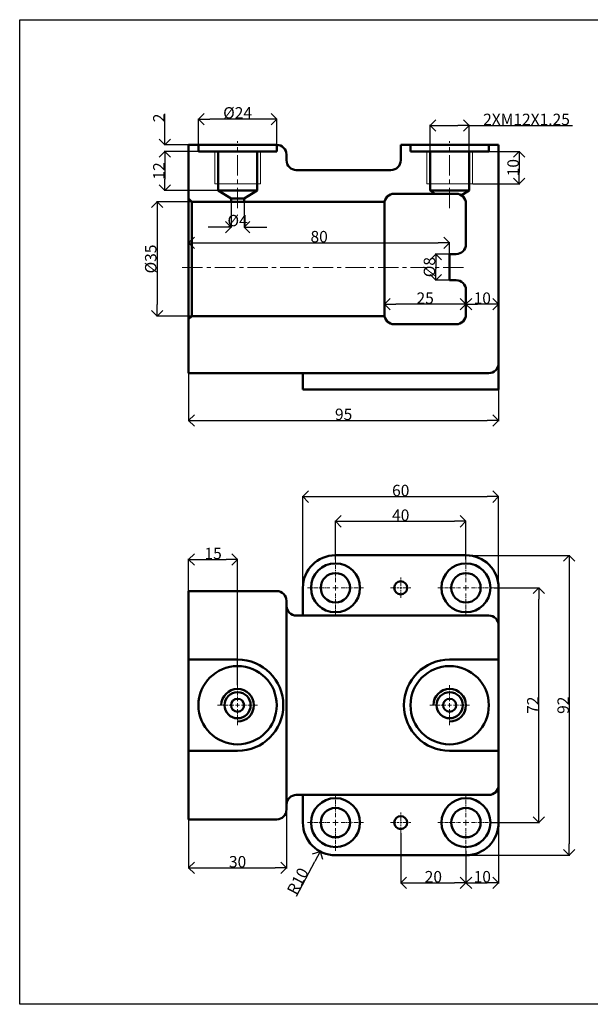
# Model space of a CAD drawing. Units: millimetres. Extents: x 47 to 397, y 26 to 328.
# Tile 1 of 2: x 47 to 222, y 26 to 328. Entities that reach past the tile are written whole.
import ezdxf

# ---------------------------------------------------------------- set-up
doc = ezdxf.new("R2010")
doc.units = ezdxf.units.MM
doc.header["$MEASUREMENT"] = 0
doc.linetypes.add('CENTER', pattern=[2, 1.25, -0.25, 0.25, -0.25])
for name, color, linetype, lineweight in [('M-CNTR', 1, 'CENTER', 18), ('M-DIMS', 2, 'Continuous', 25), ('M-OUTL', 7, 'Continuous', 50), ('M-THRD', 8, 'Continuous', 18), ('M-TTLB', 7, 'Continuous', 25)]:
    doc.layers.add(name, color=color, linetype=linetype, lineweight=lineweight)
doc.styles.get("Standard").update_dxf_attribs({"font": 'arial.ttf'})
doc.dimstyles.get("Standard").update_dxf_attribs({"dimtxt": 3.5, "dimasz": 3.5, "dimexe": 0.18, "dimexo": 0.0625, "dimgap": 0.09, "dimtad": 1, "dimdec": 0, "dimzin": 0, "dimdsep": 46, "dimtxsty": 'Standard', "dimblk": 'OPEN90', "dimcen": 0.09, "dimclre": 251, "dimadec": 0, "dimazin": 0, "dimtfac": 1, "dimtdec": 0, "dimtofl": 0, "dimtmove": 0, "dimatfit": 3, "dimfxl": 1, "dimtolj": 1, "dimtzin": 0, "dimarcsym": 0})

# ---------------------------------------------------------------- blocks, each defined once
blk = doc.blocks.new('*U2')
at = {"layer": 'M-CNTR', "color": 0, "transparency": 16777216}
for p, q in [((0, 1.2), (0, 6.12)), ((-6.12, 0), (-1.2, 0)), ((1.2, 0), (6.12, 0)), ((0, -6.12), (0, -1.2))]:
    blk.add_line(p, q, dxfattribs=at)
at = {"layer": 'M-CNTR', "color": 0, "linetype": 'Continuous', "transparency": 16777216}
for p, q in [((-0.6, 0), (0.6, 0)), ((0, -0.6), (0, 0.6))]:
    blk.add_line(p, q, dxfattribs=at)
blk = doc.blocks.new('*U3')
at = {"layer": 'M-CNTR', "color": 0, "transparency": 16777216}
for p, q in [((0, 1.2), (0, 6.12)), ((-6.12, 0), (-1.2, 0)), ((1.2, 0), (6.12, 0)), ((0, -6.12), (0, -1.2))]:
    blk.add_line(p, q, dxfattribs=at)
at = {"layer": 'M-CNTR', "color": 0, "linetype": 'Continuous', "transparency": 16777216}
for p, q in [((-0.6, 0), (0.6, 0)), ((0, -0.6), (0, 0.6))]:
    blk.add_line(p, q, dxfattribs=at)
blk = doc.blocks.new('*U4')
at = {"layer": 'M-CNTR', "color": 0, "transparency": 16777216}
for p, q in [((0, 1.7), (0, 8.62)), ((-8.62, 0), (-1.7, 0)), ((1.7, 0), (8.62, 0)), ((0, -8.62), (0, -1.7))]:
    blk.add_line(p, q, dxfattribs=at)
at = {"layer": 'M-CNTR', "color": 0, "linetype": 'Continuous', "transparency": 16777216}
for p, q in [((-0.85, 0), (0.85, 0)), ((0, -0.85), (0, 0.85))]:
    blk.add_line(p, q, dxfattribs=at)
blk = doc.blocks.new('*U5')
at = {"layer": 'M-CNTR', "color": 0, "transparency": 16777216}
for p, q in [((0, 1.7), (0, 8.62)), ((-8.62, 0), (-1.7, 0)), ((1.7, 0), (8.62, 0)), ((0, -8.62), (0, -1.7))]:
    blk.add_line(p, q, dxfattribs=at)
at = {"layer": 'M-CNTR', "color": 0, "linetype": 'Continuous', "transparency": 16777216}
for p, q in [((-0.85, 0), (0.85, 0)), ((0, -0.85), (0, 0.85))]:
    blk.add_line(p, q, dxfattribs=at)
blk = doc.blocks.new('*U6')
at = {"layer": 'M-CNTR', "color": 0, "transparency": 16777216}
for p, q in [((0, 0.6), (0, 3.12)), ((-3.12, 0), (-0.6, 0)), ((0.6, 0), (3.12, 0)), ((0, -3.12), (0, -0.6))]:
    blk.add_line(p, q, dxfattribs=at)
at = {"layer": 'M-CNTR', "color": 0, "linetype": 'Continuous', "transparency": 16777216}
for p, q in [((-0.3, 0), (0.3, 0)), ((0, -0.3), (0, 0.3))]:
    blk.add_line(p, q, dxfattribs=at)
blk = doc.blocks.new('*U9')
at = {"layer": 'M-CNTR', "color": 0, "transparency": 16777216}
for p, q in [((0, 1.7), (0, 8.62)), ((-8.62, 0), (-1.7, 0)), ((1.7, 0), (8.62, 0)), ((0, -8.62), (0, -1.7))]:
    blk.add_line(p, q, dxfattribs=at)
at = {"layer": 'M-CNTR', "color": 0, "linetype": 'Continuous', "transparency": 16777216}
for p, q in [((-0.85, 0), (0.85, 0)), ((0, -0.85), (0, 0.85))]:
    blk.add_line(p, q, dxfattribs=at)
blk = doc.blocks.new('*U7')
at = {"layer": 'M-CNTR', "color": 0, "transparency": 16777216}
for p, q in [((0, 1.7), (0, 8.62)), ((-8.62, 0), (-1.7, 0)), ((1.7, 0), (8.62, 0)), ((0, -8.62), (0, -1.7))]:
    blk.add_line(p, q, dxfattribs=at)
at = {"layer": 'M-CNTR', "color": 0, "linetype": 'Continuous', "transparency": 16777216}
for p, q in [((-0.85, 0), (0.85, 0)), ((0, -0.85), (0, 0.85))]:
    blk.add_line(p, q, dxfattribs=at)
blk = doc.blocks.new('*U8')
at = {"layer": 'M-CNTR', "color": 0, "transparency": 16777216}
for p, q in [((0, 0.6), (0, 3.12)), ((-3.12, 0), (-0.6, 0)), ((0.6, 0), (3.12, 0)), ((0, -3.12), (0, -0.6))]:
    blk.add_line(p, q, dxfattribs=at)
at = {"layer": 'M-CNTR', "color": 0, "linetype": 'Continuous', "transparency": 16777216}
for p, q in [((-0.3, 0), (0.3, 0)), ((0, -0.3), (0, 0.3))]:
    blk.add_line(p, q, dxfattribs=at)
blk = doc.blocks.new('_Open90')
at = {"color": 0, "linetype": 'ByBlock', "lineweight": -2}
for p, q in [((0, 0), (-1, 0)), ((-0.5, 0.5), (0, 0)), ((0, 0), (-0.5, -0.5))]:
    blk.add_line(p, q, dxfattribs=at)
blk = doc.blocks.new('*D10')
at = {"layer": 'Defpoints', "color": 0, "transparency": 16777216}
for p in [(101.94, 297.85), (101.94, 290.01), (125.94, 290.01)]:
    blk.add_point(p, dxfattribs=at)
at = {"layer": 'M-DIMS', "color": 0, "lineweight": -2, "transparency": 16777216}
for p, q in [((101.94, 290.07), (101.94, 298.03)), ((122.44, 297.85), (105.44, 297.85)), ((125.94, 290.07), (125.94, 298.03))]:
    blk.add_line(p, q, dxfattribs=at)
at = {"layer": 'M-DIMS', "color": 0, "lineweight": -2, "transparency": 16777216, "xscale": 3.5, "yscale": 3.5, "zscale": 3.5, "rotation": 180}
blk.add_blockref('_Open90', (101.94, 297.85), dxfattribs=at)
at = {"layer": 'M-DIMS', "color": 0, "lineweight": -2, "transparency": 16777216, "xscale": 3.5, "yscale": 3.5, "zscale": 3.5}
blk.add_blockref('_Open90', (125.94, 297.85), dxfattribs=at)
at = {"layer": 'M-DIMS', "color": 0, "transparency": 16777216, "insert": (113.94, 299.82), "char_height": 3.5, "attachment_point": 5}
blk.add_mtext('\\A1;%%C24', dxfattribs=at)
blk = doc.blocks.new('*D11')
at = {"layer": 'Defpoints', "color": 0, "transparency": 16777216}
for p in [(91.65, 290.01), (98.94, 290.01), (101.94, 288.01)]:
    blk.add_point(p, dxfattribs=at)
at = {"layer": 'M-DIMS', "color": 0, "lineweight": -2, "transparency": 16777216}
for p, q in [((91.65, 293.51), (91.65, 299.51)), ((98.88, 290.01), (91.47, 290.01)), ((101.88, 288.01), (91.47, 288.01)), ((91.65, 284.51), (91.65, 281.01))]:
    blk.add_line(p, q, dxfattribs=at)
at = {"layer": 'M-DIMS', "color": 0, "lineweight": -2, "transparency": 16777216, "xscale": 3.5, "yscale": 3.5, "zscale": 3.5}
for p, rotation in [((91.65, 290.01), 270), ((91.65, 288.01), 90)]:
    blk.add_blockref('_Open90', p, dxfattribs=dict(at, rotation=rotation))
at = {"layer": 'M-DIMS', "color": 0, "transparency": 16777216, "insert": (89.8, 298.26), "char_height": 3.5, "attachment_point": 5, "rotation": 90}
blk.add_mtext('\\A1;2', dxfattribs=at)
blk = doc.blocks.new('*D12')
at = {"layer": 'Defpoints', "color": 0, "transparency": 16777216}
for p in [(101.94, 288.01), (91.65, 276.01), (107.94, 276.01)]:
    blk.add_point(p, dxfattribs=at)
at = {"layer": 'M-DIMS', "color": 0, "lineweight": -2, "transparency": 16777216}
for p, q in [((101.88, 288.01), (91.47, 288.01)), ((91.65, 284.51), (91.65, 279.51)), ((107.88, 276.01), (91.47, 276.01))]:
    blk.add_line(p, q, dxfattribs=at)
at = {"layer": 'M-DIMS', "color": 0, "lineweight": -2, "transparency": 16777216, "xscale": 3.5, "yscale": 3.5, "zscale": 3.5}
for p, rotation in [((91.65, 288.01), 90), ((91.65, 276.01), 270)]:
    blk.add_blockref('_Open90', p, dxfattribs=dict(at, rotation=rotation))
at = {"layer": 'M-DIMS', "color": 0, "transparency": 16777216, "insert": (89.8, 282.01), "char_height": 3.5, "attachment_point": 5, "rotation": 90}
blk.add_mtext('\\A1;12', dxfattribs=at)
blk = doc.blocks.new('*D13')
at = {"layer": 'Defpoints', "color": 0, "transparency": 16777216}
for p in [(111.94, 272.51), (115.94, 272.51), (111.94, 264.8)]:
    blk.add_point(p, dxfattribs=at)
at = {"layer": 'M-DIMS', "color": 0, "lineweight": -2, "transparency": 16777216}
for p, q in [((111.94, 272.45), (111.94, 264.62)), ((115.94, 272.45), (115.94, 264.62)), ((108.44, 264.8), (104.94, 264.8)), ((119.44, 264.8), (122.94, 264.8))]:
    blk.add_line(p, q, dxfattribs=at)
at = {"layer": 'M-DIMS', "color": 0, "lineweight": -2, "transparency": 16777216, "xscale": 3.5, "yscale": 3.5, "zscale": 3.5}
blk.add_blockref('_Open90', (111.94, 264.8), dxfattribs=at)
at = {"layer": 'M-DIMS', "color": 0, "lineweight": -2, "transparency": 16777216, "xscale": 3.5, "yscale": 3.5, "zscale": 3.5, "rotation": 180}
blk.add_blockref('_Open90', (115.94, 264.8), dxfattribs=at)
at = {"layer": 'M-DIMS', "color": 0, "transparency": 16777216, "insert": (113.94, 266.78), "char_height": 3.5, "attachment_point": 5}
blk.add_mtext('\\A1;%%C4', dxfattribs=at)
blk = doc.blocks.new('*D14')
at = {"layer": 'Defpoints', "color": 0, "transparency": 16777216}
for p in [(99.94, 272.51), (89.29, 237.51), (99.94, 237.51)]:
    blk.add_point(p, dxfattribs=at)
at = {"layer": 'M-DIMS', "color": 0, "lineweight": -2, "transparency": 16777216}
for p, q in [((99.88, 272.51), (89.11, 272.51)), ((89.29, 269.01), (89.29, 241.01)), ((99.88, 237.51), (89.11, 237.51))]:
    blk.add_line(p, q, dxfattribs=at)
at = {"layer": 'M-DIMS', "color": 0, "lineweight": -2, "transparency": 16777216, "xscale": 3.5, "yscale": 3.5, "zscale": 3.5}
for p, rotation in [((89.29, 272.51), 90), ((89.29, 237.51), 270)]:
    blk.add_blockref('_Open90', p, dxfattribs=dict(at, rotation=rotation))
at = {"layer": 'M-DIMS', "color": 0, "transparency": 16777216, "insert": (87.31, 255.01), "char_height": 3.5, "attachment_point": 5, "rotation": 90}
blk.add_mtext('\\A1;%%C35', dxfattribs=at)
blk = doc.blocks.new('*D15')
at = {"layer": 'Defpoints', "color": 0, "transparency": 16777216}
for p in [(98.94, 220.01), (193.94, 215.01), (193.94, 205.49)]:
    blk.add_point(p, dxfattribs=at)
at = {"layer": 'M-DIMS', "color": 0, "lineweight": -2, "transparency": 16777216}
for p, q in [((98.94, 219.95), (98.94, 205.31)), ((193.94, 214.95), (193.94, 205.31)), ((102.44, 205.49), (190.44, 205.49))]:
    blk.add_line(p, q, dxfattribs=at)
at = {"layer": 'M-DIMS', "color": 0, "lineweight": -2, "transparency": 16777216, "xscale": 3.5, "yscale": 3.5, "zscale": 3.5, "rotation": 180}
blk.add_blockref('_Open90', (98.94, 205.49), dxfattribs=at)
at = {"layer": 'M-DIMS', "color": 0, "lineweight": -2, "transparency": 16777216, "xscale": 3.5, "yscale": 3.5, "zscale": 3.5}
blk.add_blockref('_Open90', (193.94, 205.49), dxfattribs=at)
at = {"layer": 'M-DIMS', "color": 0, "transparency": 16777216, "insert": (146.44, 207.37), "char_height": 3.5, "attachment_point": 5}
blk.add_mtext('\\A1;95', dxfattribs=at)
blk = doc.blocks.new('*D16')
at = {"layer": 'Defpoints', "color": 0, "transparency": 16777216}
for p in [(183.94, 241.12), (183.94, 241.12), (193.94, 241.12)]:
    blk.add_point(p, dxfattribs=at)
at = {"layer": 'M-DIMS', "color": 0, "lineweight": -2, "transparency": 16777216}
for p, q in [((183.94, 241.19), (183.94, 241.3)), ((190.44, 241.12), (187.44, 241.12)), ((193.94, 241.19), (193.94, 241.3))]:
    blk.add_line(p, q, dxfattribs=at)
at = {"layer": 'M-DIMS', "color": 0, "lineweight": -2, "transparency": 16777216, "xscale": 3.5, "yscale": 3.5, "zscale": 3.5, "rotation": 180}
blk.add_blockref('_Open90', (183.94, 241.12), dxfattribs=at)
at = {"layer": 'M-DIMS', "color": 0, "lineweight": -2, "transparency": 16777216, "xscale": 3.5, "yscale": 3.5, "zscale": 3.5}
blk.add_blockref('_Open90', (193.94, 241.12), dxfattribs=at)
at = {"layer": 'M-DIMS', "color": 0, "transparency": 16777216, "insert": (188.94, 243), "char_height": 3.5, "attachment_point": 5}
blk.add_mtext('\\A1;10', dxfattribs=at)
blk = doc.blocks.new('*D17')
at = {"layer": 'Defpoints', "color": 0, "transparency": 16777216}
for p in [(158.94, 241.12), (158.94, 241.12), (183.94, 241.12)]:
    blk.add_point(p, dxfattribs=at)
at = {"layer": 'M-DIMS', "color": 0, "lineweight": -2, "transparency": 16777216}
for p, q in [((158.94, 241.19), (158.94, 241.3)), ((180.44, 241.12), (162.44, 241.12)), ((183.94, 241.19), (183.94, 241.3))]:
    blk.add_line(p, q, dxfattribs=at)
at = {"layer": 'M-DIMS', "color": 0, "lineweight": -2, "transparency": 16777216, "xscale": 3.5, "yscale": 3.5, "zscale": 3.5, "rotation": 180}
blk.add_blockref('_Open90', (158.94, 241.12), dxfattribs=at)
at = {"layer": 'M-DIMS', "color": 0, "lineweight": -2, "transparency": 16777216, "xscale": 3.5, "yscale": 3.5, "zscale": 3.5}
blk.add_blockref('_Open90', (183.94, 241.12), dxfattribs=at)
at = {"layer": 'M-DIMS', "color": 0, "transparency": 16777216, "insert": (171.44, 243), "char_height": 3.5, "attachment_point": 5}
blk.add_mtext('\\A1;25', dxfattribs=at)
blk = doc.blocks.new('*D18')
at = {"layer": 'Defpoints', "color": 0, "transparency": 16777216}
for p in [(178.94, 256.51), (174.72, 248.51), (178.94, 248.51)]:
    blk.add_point(p, dxfattribs=at)
at = {"layer": 'M-DIMS', "color": 0, "lineweight": -2, "transparency": 16777216}
for p, q in [((178.88, 256.51), (174.54, 256.51)), ((174.72, 253.01), (174.72, 252.01)), ((178.88, 248.51), (174.54, 248.51))]:
    blk.add_line(p, q, dxfattribs=at)
at = {"layer": 'M-DIMS', "color": 0, "lineweight": -2, "transparency": 16777216, "xscale": 3.5, "yscale": 3.5, "zscale": 3.5}
for p, rotation in [((174.72, 256.51), 90), ((174.72, 248.51), 270)]:
    blk.add_blockref('_Open90', p, dxfattribs=dict(at, rotation=rotation))
at = {"layer": 'M-DIMS', "color": 0, "transparency": 16777216, "insert": (172.74, 252.51), "char_height": 3.5, "attachment_point": 5, "rotation": 90}
blk.add_mtext('\\A1;%%C8', dxfattribs=at)
blk = doc.blocks.new('*D19')
at = {"layer": 'Defpoints', "color": 0, "transparency": 16777216}
for p in [(98.94, 261.88), (178.94, 259.98), (178.94, 256.51)]:
    blk.add_point(p, dxfattribs=at)
at = {"layer": 'M-DIMS', "color": 0, "lineweight": -2, "transparency": 16777216}
for p, q in [((98.94, 261.81), (98.94, 259.8)), ((102.44, 259.98), (175.44, 259.98)), ((178.94, 256.57), (178.94, 260.16))]:
    blk.add_line(p, q, dxfattribs=at)
at = {"layer": 'M-DIMS', "color": 0, "lineweight": -2, "transparency": 16777216, "xscale": 3.5, "yscale": 3.5, "zscale": 3.5, "rotation": 180}
blk.add_blockref('_Open90', (98.94, 259.98), dxfattribs=at)
at = {"layer": 'M-DIMS', "color": 0, "lineweight": -2, "transparency": 16777216, "xscale": 3.5, "yscale": 3.5, "zscale": 3.5}
blk.add_blockref('_Open90', (178.94, 259.98), dxfattribs=at)
at = {"layer": 'M-DIMS', "color": 0, "transparency": 16777216, "insert": (138.94, 261.86), "char_height": 3.5, "attachment_point": 5}
blk.add_mtext('\\A1;80', dxfattribs=at)
blk = doc.blocks.new('*D20')
at = {"layer": 'Defpoints', "color": 0, "transparency": 16777216}
for p in [(184.94, 295.93), (172.94, 288.01), (184.94, 288.01)]:
    blk.add_point(p, dxfattribs=at)
at = {"layer": 'M-DIMS', "color": 0, "lineweight": -2, "transparency": 16777216}
for p, q in [((172.94, 288.07), (172.94, 296.11)), ((176.44, 295.93), (181.44, 295.93)), ((184.94, 288.07), (184.94, 296.11)), ((184.94, 295.93), (216.55, 295.93))]:
    blk.add_line(p, q, dxfattribs=at)
at = {"layer": 'M-DIMS', "color": 0, "lineweight": -2, "transparency": 16777216, "xscale": 3.5, "yscale": 3.5, "zscale": 3.5, "rotation": 180}
blk.add_blockref('_Open90', (172.94, 295.93), dxfattribs=at)
at = {"layer": 'M-DIMS', "color": 0, "lineweight": -2, "transparency": 16777216, "xscale": 3.5, "yscale": 3.5, "zscale": 3.5}
blk.add_blockref('_Open90', (184.94, 295.93), dxfattribs=at)
at = {"layer": 'M-DIMS', "color": 0, "transparency": 16777216, "insert": (202.5, 297.81), "char_height": 3.5, "attachment_point": 5}
blk.add_mtext('\\A1;2XM12X1.25', dxfattribs=at)
blk = doc.blocks.new('*D21')
at = {"layer": 'Defpoints', "color": 0, "transparency": 16777216}
for p in [(190.94, 288.01), (185.94, 278.01), (200.25, 278.01)]:
    blk.add_point(p, dxfattribs=at)
at = {"layer": 'M-DIMS', "color": 0, "lineweight": -2, "transparency": 16777216}
for p, q in [((191.01, 288.01), (200.43, 288.01)), ((200.25, 284.51), (200.25, 281.51)), ((186.01, 278.01), (200.43, 278.01))]:
    blk.add_line(p, q, dxfattribs=at)
at = {"layer": 'M-DIMS', "color": 0, "lineweight": -2, "transparency": 16777216, "xscale": 3.5, "yscale": 3.5, "zscale": 3.5}
for p, rotation in [((200.25, 288.01), 90), ((200.25, 278.01), 270)]:
    blk.add_blockref('_Open90', p, dxfattribs=dict(at, rotation=rotation))
at = {"layer": 'M-DIMS', "color": 0, "transparency": 16777216, "insert": (198.38, 283.01), "char_height": 3.5, "attachment_point": 5, "rotation": 90}
blk.add_mtext('\\A1;10', dxfattribs=at)
blk = doc.blocks.new('*D34')
at = {"layer": 'Defpoints', "color": 0, "transparency": 16777216}
for p in [(113.94, 162.84), (98.94, 153.18), (113.94, 124.3)]:
    blk.add_point(p, dxfattribs=at)
at = {"layer": 'M-DIMS', "color": 0, "lineweight": -2, "transparency": 16777216}
for p, q in [((98.94, 153.24), (98.94, 163.02)), ((102.44, 162.84), (110.44, 162.84)), ((113.94, 124.36), (113.94, 163.02))]:
    blk.add_line(p, q, dxfattribs=at)
at = {"layer": 'M-DIMS', "color": 0, "lineweight": -2, "transparency": 16777216, "xscale": 3.5, "yscale": 3.5, "zscale": 3.5, "rotation": 180}
blk.add_blockref('_Open90', (98.94, 162.84), dxfattribs=at)
at = {"layer": 'M-DIMS', "color": 0, "lineweight": -2, "transparency": 16777216, "xscale": 3.5, "yscale": 3.5, "zscale": 3.5}
blk.add_blockref('_Open90', (113.94, 162.84), dxfattribs=at)
at = {"layer": 'M-DIMS', "color": 0, "transparency": 16777216, "insert": (106.44, 164.72), "char_height": 3.5, "attachment_point": 5}
blk.add_mtext('\\A1;15', dxfattribs=at)
blk = doc.blocks.new('*D35')
at = {"layer": 'Defpoints', "color": 0, "transparency": 16777216}
for p in [(128.94, 87.68), (98.94, 83.18), (128.94, 68.31)]:
    blk.add_point(p, dxfattribs=at)
at = {"layer": 'M-DIMS', "color": 0, "lineweight": -2, "transparency": 16777216}
for p, q in [((128.94, 87.61), (128.94, 68.13)), ((98.94, 83.11), (98.94, 68.13)), ((102.44, 68.31), (125.44, 68.31))]:
    blk.add_line(p, q, dxfattribs=at)
at = {"layer": 'M-DIMS', "color": 0, "lineweight": -2, "transparency": 16777216, "xscale": 3.5, "yscale": 3.5, "zscale": 3.5, "rotation": 180}
blk.add_blockref('_Open90', (98.94, 68.31), dxfattribs=at)
at = {"layer": 'M-DIMS', "color": 0, "lineweight": -2, "transparency": 16777216, "xscale": 3.5, "yscale": 3.5, "zscale": 3.5}
blk.add_blockref('_Open90', (128.94, 68.31), dxfattribs=at)
at = {"layer": 'M-DIMS', "color": 0, "transparency": 16777216, "insert": (113.94, 70.18), "char_height": 3.5, "attachment_point": 5}
blk.add_mtext('\\A1;30', dxfattribs=at)
blk = doc.blocks.new('*D36')
at = {"layer": 'Defpoints', "color": 0, "transparency": 16777216}
for p in [(143.94, 82.18), (139.28, 73.33)]:
    blk.add_point(p, dxfattribs=at)
at = {"layer": 'M-DIMS', "color": 0, "lineweight": -2, "transparency": 16777216}
for p, q in [((143.85, 82.18), (144.03, 82.18)), ((143.94, 82.09), (143.94, 82.27)), ((132.04, 59.59), (137.65, 70.23))]:
    blk.add_line(p, q, dxfattribs=at)
at = {"layer": 'M-DIMS', "color": 0, "lineweight": -2, "transparency": 16777216, "xscale": 3.5, "yscale": 3.5, "zscale": 3.5, "rotation": 62.1981860679944}
blk.add_blockref('_Open90', (139.28, 73.33), dxfattribs=at)
at = {"layer": 'M-DIMS', "color": 0, "transparency": 16777216, "insert": (132.37, 64.24), "char_height": 3.5, "attachment_point": 5, "rotation": 62.1982}
blk.add_mtext('\\A1;R10', dxfattribs=at)
blk = doc.blocks.new('*D37')
at = {"layer": 'Defpoints', "color": 0, "transparency": 16777216}
for p in [(163.94, 79.06), (183.94, 73.56), (183.94, 63.72)]:
    blk.add_point(p, dxfattribs=at)
at = {"layer": 'M-DIMS', "color": 0, "lineweight": -2, "transparency": 16777216}
for p, q in [((163.94, 78.99), (163.94, 63.54)), ((183.94, 73.49), (183.94, 63.54)), ((167.44, 63.72), (180.44, 63.72))]:
    blk.add_line(p, q, dxfattribs=at)
at = {"layer": 'M-DIMS', "color": 0, "lineweight": -2, "transparency": 16777216, "xscale": 3.5, "yscale": 3.5, "zscale": 3.5, "rotation": 180}
blk.add_blockref('_Open90', (163.94, 63.72), dxfattribs=at)
at = {"layer": 'M-DIMS', "color": 0, "lineweight": -2, "transparency": 16777216, "xscale": 3.5, "yscale": 3.5, "zscale": 3.5}
blk.add_blockref('_Open90', (183.94, 63.72), dxfattribs=at)
at = {"layer": 'M-DIMS', "color": 0, "transparency": 16777216, "insert": (173.94, 65.6), "char_height": 3.5, "attachment_point": 5}
blk.add_mtext('\\A1;20', dxfattribs=at)
blk = doc.blocks.new('*D38')
at = {"layer": 'Defpoints', "color": 0, "transparency": 16777216}
for p in [(193.94, 82.18), (183.94, 73.56), (193.94, 63.72)]:
    blk.add_point(p, dxfattribs=at)
at = {"layer": 'M-DIMS', "color": 0, "lineweight": -2, "transparency": 16777216}
for p, q in [((193.94, 82.11), (193.94, 63.54)), ((183.94, 73.49), (183.94, 63.54)), ((187.44, 63.72), (190.44, 63.72))]:
    blk.add_line(p, q, dxfattribs=at)
at = {"layer": 'M-DIMS', "color": 0, "lineweight": -2, "transparency": 16777216, "xscale": 3.5, "yscale": 3.5, "zscale": 3.5, "rotation": 180}
blk.add_blockref('_Open90', (183.94, 63.72), dxfattribs=at)
at = {"layer": 'M-DIMS', "color": 0, "lineweight": -2, "transparency": 16777216, "xscale": 3.5, "yscale": 3.5, "zscale": 3.5}
blk.add_blockref('_Open90', (193.94, 63.72), dxfattribs=at)
at = {"layer": 'M-DIMS', "color": 0, "transparency": 16777216, "insert": (188.94, 65.6), "char_height": 3.5, "attachment_point": 5}
blk.add_mtext('\\A1;10', dxfattribs=at)
blk = doc.blocks.new('*D39')
at = {"layer": 'Defpoints', "color": 0, "transparency": 16777216}
for p in [(192.56, 154.18), (206.27, 154.18), (191.44, 82.18)]:
    blk.add_point(p, dxfattribs=at)
at = {"layer": 'M-DIMS', "color": 0, "lineweight": -2, "transparency": 16777216}
for p, q in [((192.63, 154.18), (206.45, 154.18)), ((206.27, 85.68), (206.27, 150.68)), ((191.51, 82.18), (206.45, 82.18))]:
    blk.add_line(p, q, dxfattribs=at)
at = {"layer": 'M-DIMS', "color": 0, "lineweight": -2, "transparency": 16777216, "xscale": 3.5, "yscale": 3.5, "zscale": 3.5}
for p, rotation in [((206.27, 154.18), 90), ((206.27, 82.18), 270)]:
    blk.add_blockref('_Open90', p, dxfattribs=dict(at, rotation=rotation))
at = {"layer": 'M-DIMS', "color": 0, "transparency": 16777216, "insert": (204.42, 118.18), "char_height": 3.5, "attachment_point": 5, "rotation": 90}
blk.add_mtext('\\A1;72', dxfattribs=at)
blk = doc.blocks.new('*D40')
at = {"layer": 'Defpoints', "color": 0, "transparency": 16777216}
for p in [(184.91, 164.13), (184.8, 72.21), (215.61, 72.21)]:
    blk.add_point(p, dxfattribs=at)
at = {"layer": 'M-DIMS', "color": 0, "lineweight": -2, "transparency": 16777216}
for p, q in [((184.98, 164.13), (215.79, 164.13)), ((215.61, 160.63), (215.61, 75.71)), ((184.86, 72.21), (215.79, 72.21))]:
    blk.add_line(p, q, dxfattribs=at)
at = {"layer": 'M-DIMS', "color": 0, "lineweight": -2, "transparency": 16777216, "xscale": 3.5, "yscale": 3.5, "zscale": 3.5}
for p, rotation in [((215.61, 164.13), 90), ((215.61, 72.21), 270)]:
    blk.add_blockref('_Open90', p, dxfattribs=dict(at, rotation=rotation))
at = {"layer": 'M-DIMS', "color": 0, "transparency": 16777216, "insert": (213.73, 118.17), "char_height": 3.5, "attachment_point": 5, "rotation": 90}
blk.add_mtext('\\A1;92', dxfattribs=at)
blk = doc.blocks.new('*D41')
at = {"layer": 'Defpoints', "color": 0, "transparency": 16777216}
for p in [(183.94, 174.57), (143.94, 162.8), (183.94, 162.8)]:
    blk.add_point(p, dxfattribs=at)
at = {"layer": 'M-DIMS', "color": 0, "lineweight": -2, "transparency": 16777216}
for p, q in [((143.94, 162.86), (143.94, 174.75)), ((147.44, 174.57), (180.44, 174.57)), ((183.94, 162.86), (183.94, 174.75))]:
    blk.add_line(p, q, dxfattribs=at)
at = {"layer": 'M-DIMS', "color": 0, "lineweight": -2, "transparency": 16777216, "xscale": 3.5, "yscale": 3.5, "zscale": 3.5, "rotation": 180}
blk.add_blockref('_Open90', (143.94, 174.57), dxfattribs=at)
at = {"layer": 'M-DIMS', "color": 0, "lineweight": -2, "transparency": 16777216, "xscale": 3.5, "yscale": 3.5, "zscale": 3.5}
blk.add_blockref('_Open90', (183.94, 174.57), dxfattribs=at)
at = {"layer": 'M-DIMS', "color": 0, "transparency": 16777216, "insert": (163.94, 176.45), "char_height": 3.5, "attachment_point": 5}
blk.add_mtext('\\A1;40', dxfattribs=at)
blk = doc.blocks.new('*D42')
at = {"layer": 'Defpoints', "color": 0, "transparency": 16777216}
for p in [(193.94, 182.14), (133.94, 154.18), (193.94, 154.18)]:
    blk.add_point(p, dxfattribs=at)
at = {"layer": 'M-DIMS', "color": 0, "lineweight": -2, "transparency": 16777216}
for p, q in [((133.94, 154.24), (133.94, 182.32)), ((137.44, 182.14), (190.44, 182.14)), ((193.94, 154.24), (193.94, 182.32))]:
    blk.add_line(p, q, dxfattribs=at)
at = {"layer": 'M-DIMS', "color": 0, "lineweight": -2, "transparency": 16777216, "xscale": 3.5, "yscale": 3.5, "zscale": 3.5, "rotation": 180}
blk.add_blockref('_Open90', (133.94, 182.14), dxfattribs=at)
at = {"layer": 'M-DIMS', "color": 0, "lineweight": -2, "transparency": 16777216, "xscale": 3.5, "yscale": 3.5, "zscale": 3.5}
blk.add_blockref('_Open90', (193.94, 182.14), dxfattribs=at)
at = {"layer": 'M-DIMS', "color": 0, "transparency": 16777216, "insert": (163.94, 184.02), "char_height": 3.5, "attachment_point": 5}
blk.add_mtext('\\A1;60', dxfattribs=at)

msp = doc.modelspace()

# ---------------------------------------------------------------- linework, layer by layer
at = {"layer": 'M-CNTR', "ltscale": 5}
for p, q in [((113.94, 270.59), (113.94, 291.15)), ((178.94, 270.59), (178.94, 291.15)), ((183.23, 252.42), (95.79, 252.42))]:
    msp.add_line(p, q, dxfattribs=at)
at = {"layer": 'M-OUTL'}
for p, q in [((98.94, 290.01), (125.94, 290.01)), ((98.94, 290.01), (98.94, 220.01)), ((101.94, 288.01), (101.94, 290.01)), ((125.94, 288.01), (125.94, 290.01)), ((163.94, 290.01), (163.94, 285.27)), ((163.94, 290.01), (193.94, 290.01)), ((166.94, 288.01), (166.94, 290.01)), ((190.94, 288.01), (190.94, 290.01)), ((193.94, 290.01), (193.94, 215.01)), ((101.94, 288.01), (125.94, 288.01)), ((107.94, 276.01), (107.94, 288.01)), ((119.94, 276.01), (119.94, 288.01)), ((128.94, 287.01), (128.94, 285.27)), ((166.94, 288.01), (190.94, 288.01)), ((172.94, 276.01), (172.94, 288.01)), ((184.94, 276.01), (184.94, 288.01)), ((131.94, 282.27), (160.94, 282.27)), ((107.94, 276.01), (119.94, 276.01)), ((107.94, 276.01), (111.94, 273.51)), ((115.94, 273.51), (119.94, 276.01)), ((161.94, 275.01), (180.94, 275.01)), ((172.94, 276.01), (184.94, 276.01)), ((172.94, 276.01), (174.54, 275.01)), ((182.57, 274.53), (184.94, 276.01)), ((99.94, 272.51), (98.94, 273.51)), ((158.94, 272.51), (99.94, 272.51)), ((99.94, 272.51), (99.94, 237.51)), ((111.94, 272.51), (111.94, 273.51)), ((115.94, 273.51), (111.94, 273.51)), ((115.94, 272.51), (115.94, 273.51)), ((158.94, 272.01), (158.94, 238.01)), ((183.94, 272.01), (183.94, 259.51)), ((178.94, 256.51), (178.94, 248.51)), ((180.94, 256.51), (178.94, 256.51)), ((180.94, 248.51), (178.94, 248.51)), ((183.94, 245.51), (183.94, 238.01)), ((98.94, 236.51), (99.94, 237.51)), ((158.94, 237.51), (99.94, 237.51)), ((161.94, 235.01), (180.94, 235.01)), ((98.94, 220.01), (190.94, 220.01)), ((133.94, 215.01), (133.94, 220.01)), ((193.94, 215.01), (133.94, 215.01)), ((143.94, 164.18), (183.94, 164.18)), ((133.94, 154.18), (133.94, 145.68)), ((193.94, 154.18), (193.94, 82.18)), ((98.94, 153.18), (98.94, 83.18)), ((98.94, 153.18), (125.94, 153.18)), ((128.94, 86.18), (128.94, 150.18)), ((190.94, 145.68), (131.94, 145.68)), ((113.94, 132.18), (98.94, 132.18)), ((178.94, 132.18), (193.94, 132.18)), ((113.94, 104.18), (98.94, 104.18)), ((178.94, 104.18), (193.94, 104.18)), ((190.94, 90.68), (131.94, 90.68)), ((133.94, 90.68), (133.94, 82.18)), ((98.94, 83.18), (125.94, 83.18)), ((183.94, 72.18), (143.94, 72.18))]:
    msp.add_line(p, q, dxfattribs=at)
for centre, radius in [((143.94, 154.18), 7.5), ((183.94, 154.18), 7.5), ((143.94, 154.18), 4.5), ((183.94, 154.18), 4.5), ((163.94, 154.18), 2), ((113.94, 118.18), 12), ((178.94, 118.18), 12), ((113.94, 118.18), 4), ((178.94, 118.18), 4), ((113.94, 118.18), 2), ((178.94, 118.18), 2), ((143.94, 82.18), 7.5), ((183.94, 82.18), 7.5), ((143.94, 82.18), 4.5), ((183.94, 82.18), 4.5), ((163.94, 82.18), 2)]:
    msp.add_circle(centre, radius, dxfattribs=at)
for centre, radius, start, end in [((125.94, 287.01), 3, 0, 90), ((131.94, 285.27), 3, 180, 270), ((160.94, 285.27), 3, 270, 0), ((161.94, 272.01), 3, 90, 180), ((180.94, 272.01), 3, 0, 90), ((180.94, 259.51), 3, 270, 0), ((180.94, 245.51), 3, 0, 90), ((161.94, 238.01), 3, 180, 270), ((180.94, 238.01), 3, 270, 0), ((190.94, 223.01), 3, 270, 0), ((143.94, 154.18), 10, 90, 180), ((183.94, 154.18), 10, 0, 90), ((125.94, 150.18), 3, 0, 90), ((131.94, 148.68), 3, 180, 270), ((190.94, 142.68), 3, 0, 90), ((113.94, 118.18), 14, 270, 90), ((178.94, 118.18), 14, 90, 270), ((113.94, 118.18), 5, 270, 180), ((178.94, 118.18), 5, 270, 180), ((190.94, 93.68), 3, 270, 0), ((131.94, 87.68), 3, 90, 180), ((125.94, 86.18), 3, 270, 0), ((143.94, 82.18), 10, 180, 270), ((183.94, 82.18), 10, 270, 0)]:
    msp.add_arc(centre, radius, start, end, dxfattribs=at)
at = {"layer": 'M-THRD', "ltscale": 8}
for p, q in [((106.94, 278.01), (106.94, 288.01)), ((120.94, 278.01), (120.94, 288.01)), ((171.94, 278.01), (171.94, 288.01)), ((185.94, 278.01), (185.94, 288.01)), ((106.94, 278.01), (120.94, 278.01)), ((171.94, 278.01), (185.94, 278.01))]:
    msp.add_line(p, q, dxfattribs=at)
at = {"layer": 'M-TTLB'}
msp.add_lwpolyline([(47.15, 328.38), (396.95, 328.38), (396.95, 26.47), (47.15, 26.47)], close=True, dxfattribs=at)

# ---------------------------------------------------------------- block references
at = {"layer": 'M-CNTR'}
for name, p in [('*U4', (143.94, 154.18)), ('*U5', (183.94, 154.18)), ('*U6', (163.94, 154.18)), ('*U2', (113.94, 118.18)), ('*U3', (178.94, 118.18)), ('*U9', (143.94, 82.18)), ('*U7', (183.94, 82.18)), ('*U8', (163.94, 82.18))]:
    msp.add_blockref(name, p, dxfattribs=at)

# ---------------------------------------------------------------- dimensions: what is measured, and where the dimension line sits
at = {"layer": 'M-DIMS'}
for base, p1, p2, text, picture, middle in [((101.94, 297.85), (125.94, 290.01), (101.94, 290.01), '%%C<>', '*D10', (113.94, 299.82)), ((184.94, 295.93), (172.94, 288.01), (184.94, 288.01), '2XM<>X1.25', '*D20', (202.5, 297.81))]:
    dim = msp.add_linear_dim(base=base, p1=p1, p2=p2, text=text, dimstyle='Standard', override={"dimclrd": 0, "dimclre": 0, "dimclrt": 0}, dxfattribs=at)
    dim.commit()
    dim.dimension.update_dxf_attribs({"geometry": picture, "text_midpoint": middle})
for base, p1, p2, picture, middle in [((91.65, 290.01), (101.94, 288.01), (98.94, 290.01), '*D11', (89.8, 298.26)), ((91.65, 276.01), (101.94, 288.01), (107.94, 276.01), '*D12', (89.8, 282.01)), ((200.25, 278.01), (190.94, 288.01), (185.94, 278.01), '*D21', (198.38, 283.01)), ((215.61, 72.21), (184.91, 164.13), (184.8, 72.21), '*D40', (213.73, 118.17)), ((206.27, 154.18), (191.44, 82.18), (192.56, 154.18), '*D39', (204.42, 118.18))]:
    dim = msp.add_linear_dim(base=base, p1=p1, p2=p2, angle=90, dimstyle='Standard', override={"dimclrd": 0, "dimclre": 0, "dimclrt": 0}, dxfattribs=at)
    dim.commit()
    dim.dimension.update_dxf_attribs({"geometry": picture, "text_midpoint": middle})
for base, p1, p2, picture, middle in [((89.29, 237.51), (99.94, 272.51), (99.94, 237.51), '*D14', (87.31, 255.01)), ((174.72, 248.51), (178.94, 256.51), (178.94, 248.51), '*D18', (172.74, 252.51))]:
    dim = msp.add_linear_dim(base=base, p1=p1, p2=p2, angle=90, text='%%C<>', dimstyle='Standard', override={"dimclrd": 0, "dimclre": 0, "dimclrt": 0}, dxfattribs=at)
    dim.commit()
    dim.dimension.update_dxf_attribs({"geometry": picture, "text_midpoint": middle})
dim = msp.add_linear_dim(base=(111.94, 264.8), p1=(115.94, 272.51), p2=(111.94, 272.51), text='%%C<>', dimstyle='Standard', override={"dimclrd": 0, "dimclre": 0, "dimclrt": 0}, dxfattribs=at)
dim.commit()
dim.dimension.update_dxf_attribs({"geometry": '*D13', "text_midpoint": (113.94, 264.8), "dimtype": 160})
for base, p1, p2, picture, middle in [((178.94, 259.98), (98.94, 261.88), (178.94, 256.51), '*D19', (138.94, 261.86)), ((158.94, 241.12), (183.94, 241.12), (158.94, 241.12), '*D17', (171.44, 243)), ((183.94, 241.12), (193.94, 241.12), (183.94, 241.12), '*D16', (188.94, 243)), ((193.94, 205.49), (98.94, 220.01), (193.94, 215.01), '*D15', (146.44, 207.37)), ((193.94, 182.14), (133.94, 154.18), (193.94, 154.18), '*D42', (163.94, 184.02)), ((183.94, 174.57), (143.94, 162.8), (183.94, 162.8), '*D41', (163.94, 176.45)), ((113.94, 162.84), (98.94, 153.18), (113.94, 124.3), '*D34', (106.44, 164.72)), ((128.94, 68.31), (98.94, 83.18), (128.94, 87.68), '*D35', (113.94, 70.18)), ((193.94, 63.72), (183.94, 73.56), (193.94, 82.18), '*D38', (188.94, 65.6)), ((183.94, 63.72), (163.94, 79.06), (183.94, 73.56), '*D37', (173.94, 65.6))]:
    dim = msp.add_linear_dim(base=base, p1=p1, p2=p2, dimstyle='Standard', override={"dimclrd": 0, "dimclre": 0, "dimclrt": 0}, dxfattribs=at)
    dim.commit()
    dim.dimension.update_dxf_attribs({"geometry": picture, "text_midpoint": middle})
dim = msp.add_radius_dim(center=(143.94, 82.18), mpoint=(139.28, 73.33), dimstyle='Standard', override={"dimclrd": 0, "dimclre": 0, "dimclrt": 0}, dxfattribs=at)
dim.commit()
dim.dimension.update_dxf_attribs({"geometry": '*D36', "text_midpoint": (132.37, 64.24)})

doc.saveas('drawing.dxf')
